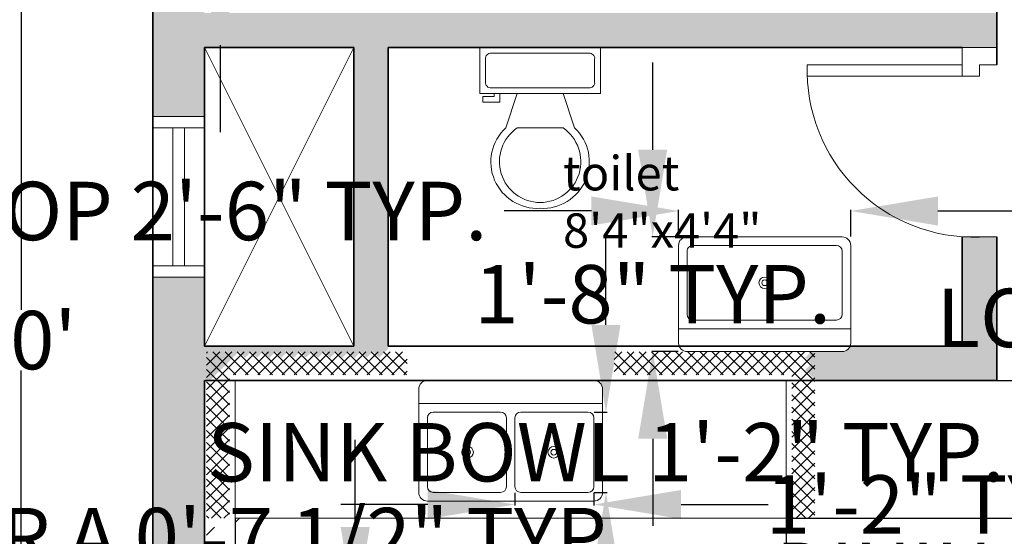
# Model space of a CAD drawing. Units: inches. Extents: x 19 to 15718, y 7 to 930.
# Tile 8 of 11: x 15243 to 15415, y 556 to 646. Entities that reach past the tile are written whole.
import ezdxf

# ---------------------------------------------------------------- set-up
doc = ezdxf.new("R2010")
doc.units = ezdxf.units.IN
doc.header["$MEASUREMENT"] = 0
for name, color, linetype, lineweight in [('A-ANNO-DIMS', 2, 'Continuous', 18), ('A-AREA-IDEN', 7, 'Continuous', 18), ('A-DOOR', 4, 'Continuous', 20), ('A-FLOR-CASE', 8, 'Continuous', 18), ('A-FLOR-CASE-PATT', 252, 'Continuous', 13), ('A-FLOR-FIXT', 9, 'Continuous', 18), ('A-FLOR-OPEN', 8, 'Continuous', 13), ('A-GLAZ', 4, 'Continuous', 18), ('A-WALL', 7, 'Continuous', 35)]:
    doc.layers.add(name, color=color, linetype=linetype, lineweight=lineweight)
doc.layers.add('A-WALL-PATT', color=18, linetype='Continuous', lineweight=13, true_color=0x000000)
doc.styles.add('Annotative', font='arial.ttf')
doc.styles.get("Standard").update_dxf_attribs({"font": 'arial.ttf'})
doc.dimstyles.get("Standard").update_dxf_attribs({"dimtxt": 10.18, "dimasz": 15.18, "dimexe": 0.18, "dimexo": 0.0625, "dimgap": 0.09, "dimtad": 0, "dimtih": 1, "dimtoh": 1, "dimdec": 0, "dimzin": 0, "dimdsep": 46, "dimlunit": 3, "dimtxsty": 'Standard', "dimcen": 0.09, "dimadec": 0, "dimazin": 0, "dimtfac": 1, "dimtdec": 0, "dimtofl": 0, "dimtmove": 0, "dimatfit": 3, "dimfxl": 1, "dimtolj": 1, "dimtzin": 0, "dimarcsym": 0})

# ---------------------------------------------------------------- blocks, each defined once
blk = doc.blocks.new('*U2')
for p, q in [((9.5, -6), (9.5, -2)), ((-10, -8.5), (-8, -8.5)), ((-10, -9.5), (-10, -8.5)), ((-8, -8.5), (-8, -8)), ((-7, -8), (-7, -9.5)), ((-4, -8), (-6, -14)), ((4, -8), (6, -14)), ((-7, -9.5), (-10, -9.5)), ((4, -14), (-4, -14))]:
    blk.add_line(p, q)
blk.add_lwpolyline([(10.5, -8), (10.5, 0), (-10.5, 0), (-10.5, -8)], close=True)
for points in [[(8.5, -1), (-8.5, -1)], [(-9.5, -2), (-9.5, -6)], [(-8.5, -7), (8.5, -7)]]:
    blk.add_lwpolyline(points)
for centre, radius, start, end in [((-8.625, -1.875), 0.8839, 81.8699, 188.1301), ((8.625, -1.875), 0.8839, 351.8699, 98.1301), ((-8.625, -6.125), 0.8839, 171.869898, 278.1301), ((8.625, -6.125), 0.8839, 261.8699, 8.1301), ((-0.4772, -19.9188), 8.0953, 133.01722, 273.38), ((0.0374, -19.8731), 7.127, 124.50543, 269.7), ((-0.0373, -19.8731), 7.127, 270.3, 55.4946), ((0.4773, -19.9188), 8.0953, 266.62, 46.9828)]:
    blk.add_arc(centre, radius, start, end)
blk = doc.blocks.new('*D17')
at = {"layer": 'A-ANNO-DIMS', "color": 0, "lineweight": -2, "transparency": 16777216}
for p, q in [((15266.62, 830.27), (15243.58, 830.27)), ((15243.76, 815.09), (15243.76, 595.52)), ((15243.76, 365.38), (15243.76, 584.95)), ((15266.62, 350.2), (15243.58, 350.2))]:
    blk.add_line(p, q, dxfattribs=at)
at = {"layer": 'A-ANNO-DIMS', "color": 0, "transparency": 16777216}
for points in [[(15241.23, 815.09), (15246.29, 815.09), (15243.76, 830.27)], [(15241.23, 365.38), (15246.29, 365.38), (15243.76, 350.2)]]:
    blk.add_solid(points, dxfattribs=at)
at = {"layer": 'Defpoints', "color": 0, "transparency": 16777216}
for p in [(15266.68, 830.27), (15243.76, 350.2), (15266.68, 350.2)]:
    blk.add_point(p, dxfattribs=at)
at = {"layer": 'A-ANNO-DIMS', "color": 0, "transparency": 16777216, "insert": (15243.76, 590.24), "char_height": 10.18, "attachment_point": 5}
blk.add_mtext("\\A1;40'", dxfattribs=at)
blk = doc.blocks.new('Sink-single - 30 in top')
blk.add_line((-15, -3.999996), (15, -3.999996))
for points in [[(-13.5, 0), (13.5, 0)], [(-15, -18.499996), (-15, -1.5)], [(15, -1.5), (15, -18.499996)], [(-13.5, -17.499996), (-13.5, -6.499996)], [(-12.5, -5.499996), (12.5, -5.499996)], [(13.5, -6.499996), (13.5, -17.499996)], [(12.5, -18.499996), (-12.5, -18.499996)], [(13.5, -19.999996), (-13.5, -19.999996)]]:
    blk.add_lwpolyline(points)
for radius in [1, 0.5]:
    blk.add_circle((0, -11.999996), radius)
for centre, radius, start, end in [((-13.5, -1.5), 1.5, 90, 180), ((13.5, -1.5), 1.5, 0, 90), ((-12.5, -6.499996), 1, 90, 180), ((12.5, -6.499996), 1, 0, 90), ((-13.5, -18.499996), 1.5, 180, 270), ((-12.5, -17.499996), 1, 180, 270), ((12.5, -17.499996), 1, 270, 0), ((13.5, -18.499996), 1.5, 270, 0)]:
    blk.add_arc(centre, radius, start, end)
blk = doc.blocks.new('DOOR-SWING-30IN')
for p, q in [((3, 6), (3, 33)), ((5, 3), (5, 33)), ((0, 6), (0, 0)), ((0, 6), (5, 6)), ((33, 6), (33, 0)), ((3, 3), (3, 0)), ((5, 3), (3, 3))]:
    blk.add_line(p, q)
blk.add_arc((4, 4), 29.02, 358.0251, 91.9749)
blk = doc.blocks.new('SINK-BOWL-14IN')
blk.add_line((0, 13), (0, 1))
for points in [[(1, 14), (12.75, 14)], [(13.75, 13), (13.75, 1)], [(12.75, 0), (1, 0)]]:
    blk.add_lwpolyline(points)
for radius in [1, 0.5]:
    blk.add_circle((6.75, 7), radius)
for centre, start, end in [((1, 13), 90, 180), ((12.75, 13), 0, 90), ((1, 1), 180, 270), ((12.75, 1), 270, 0)]:
    blk.add_arc(centre, 1, start, end)
blk = doc.blocks.new('*D40')
at = {"layer": 'A-ANNO-DIMS', "color": 0, "lineweight": -2, "transparency": 16777216}
for p, q in [((15117.25, 555.92), (15102.07, 555.92)), ((15132.43, 556.96), (15132.43, 555.74)), ((15139.78, 556.96), (15139.78, 555.74)), ((15154.96, 555.92), (15170.14, 555.92))]:
    blk.add_line(p, q, dxfattribs=at)
at = {"layer": 'A-ANNO-DIMS', "color": 0, "transparency": 16777216}
for points in [[(15117.25, 558.45), (15117.25, 553.39), (15132.43, 555.92)], [(15154.96, 558.45), (15154.96, 553.39), (15139.78, 555.92)]]:
    blk.add_solid(points, dxfattribs=at)
at = {"layer": 'Defpoints', "color": 0, "transparency": 16777216}
for p in [(15132.43, 557.02), (15139.78, 557.02), (15139.78, 555.92)]:
    blk.add_point(p, dxfattribs=at)
at = {"layer": 'A-ANNO-DIMS', "color": 0, "transparency": 16777216, "insert": (15262.49, 555.92), "char_height": 10.18, "attachment_point": 5}
blk.add_mtext('\\A1;SIDE CHAIR A 0\'-7 1/2" TYP.', dxfattribs=at)
blk = doc.blocks.new('*D42')
at = {"layer": 'A-ANNO-DIMS', "color": 0, "lineweight": -2, "transparency": 16777216}
for p, q in [((15133.17, 540.88), (15133.17, 542.1)), ((15140.52, 540.88), (15140.52, 542.1)), ((15117.99, 541.92), (15102.81, 541.92)), ((15155.7, 541.92), (15170.88, 541.92))]:
    blk.add_line(p, q, dxfattribs=at)
at = {"layer": 'A-ANNO-DIMS', "color": 0, "transparency": 16777216}
for points in [[(15117.99, 544.45), (15117.99, 539.39), (15133.17, 541.92)], [(15155.7, 544.45), (15155.7, 539.39), (15140.52, 541.92)]]:
    blk.add_solid(points, dxfattribs=at)
at = {"layer": 'Defpoints', "color": 0, "transparency": 16777216}
for p in [(15133.17, 540.82), (15140.52, 541.92), (15140.52, 540.82)]:
    blk.add_point(p, dxfattribs=at)
at = {"layer": 'A-ANNO-DIMS', "color": 0, "transparency": 16777216, "insert": (15263.22, 541.92), "char_height": 10.18, "attachment_point": 5}
blk.add_mtext('\\A1;SIDE CHAIR B 0\'-7 1/2" TYP.', dxfattribs=at)
blk = doc.blocks.new('*D46')
at = {"layer": 'A-ANNO-DIMS', "color": 0, "lineweight": -2, "transparency": 16777216}
for p, q in [((15343.07, 612.73), (15327.89, 612.73)), ((15358.25, 608.29), (15358.25, 612.91)), ((15388.25, 608.29), (15388.25, 612.91)), ((15403.43, 612.73), (15418.61, 612.73))]:
    blk.add_line(p, q, dxfattribs=at)
at = {"layer": 'A-ANNO-DIMS', "color": 0, "transparency": 16777216}
for points in [[(15343.07, 615.26), (15343.07, 610.2), (15358.25, 612.73)], [(15403.43, 615.26), (15403.43, 610.2), (15388.25, 612.73)]]:
    blk.add_solid(points, dxfattribs=at)
at = {"layer": 'Defpoints', "color": 0, "transparency": 16777216}
for p in [(15358.25, 612.73), (15358.25, 608.23), (15388.25, 608.23)]:
    blk.add_point(p, dxfattribs=at)
at = {"layer": 'A-ANNO-DIMS', "color": 0, "transparency": 16777216, "insert": (15257.09, 612.73), "char_height": 10.18, "attachment_point": 5}
blk.add_mtext('\\A1;BASIN TOP 2\'-6" TYP.', dxfattribs=at)
blk = doc.blocks.new('*D47')
at = {"layer": 'A-ANNO-DIMS', "color": 0, "lineweight": -2, "transparency": 16777216}
for p, q in [((15353.75, 623.41), (15353.75, 638.59)), ((15358.19, 608.23), (15353.57, 608.23)), ((15358.19, 588.23), (15353.57, 588.23)), ((15353.75, 573.05), (15353.75, 557.87))]:
    blk.add_line(p, q, dxfattribs=at)
at = {"layer": 'A-ANNO-DIMS', "color": 0, "transparency": 16777216}
for points in [[(15351.22, 623.41), (15356.28, 623.41), (15353.75, 608.23)], [(15351.22, 573.05), (15356.28, 573.05), (15353.75, 588.23)]]:
    blk.add_solid(points, dxfattribs=at)
at = {"layer": 'Defpoints', "color": 0, "transparency": 16777216}
for p in [(15358.25, 608.23), (15353.75, 588.23), (15358.25, 588.23)]:
    blk.add_point(p, dxfattribs=at)
at = {"layer": 'A-ANNO-DIMS', "color": 0, "transparency": 16777216, "insert": (15353.75, 598.23), "char_height": 10.18, "attachment_point": 5}
blk.add_mtext('\\A1;1\'-8" TYP.', dxfattribs=at)
blk = doc.blocks.new('*D57')
at = {"layer": 'A-ANNO-DIMS', "color": 0, "lineweight": -2, "transparency": 16777216}
for p, q in [((15165.53, 693.18), (15165.53, 708.36)), ((15165.53, 708.36), (15180.71, 708.36)), ((15166.82, 678), (15165.35, 678)), ((15166.82, 669.42), (15165.35, 669.42)), ((15165.53, 654.24), (15165.53, 639.06))]:
    blk.add_line(p, q, dxfattribs=at)
at = {"layer": 'A-ANNO-DIMS', "color": 0, "transparency": 16777216}
for points in [[(15163, 693.18), (15168.06, 693.18), (15165.53, 678)], [(15163, 654.24), (15168.06, 654.24), (15165.53, 669.42)]]:
    blk.add_solid(points, dxfattribs=at)
at = {"layer": 'Defpoints', "color": 0, "transparency": 16777216}
for p in [(15165.53, 678), (15166.88, 678), (15166.88, 669.42)]:
    blk.add_point(p, dxfattribs=at)
at = {"layer": 'A-ANNO-DIMS', "color": 0, "transparency": 16777216, "insert": (15223.69, 708.36), "char_height": 10.18, "attachment_point": 5}
blk.add_mtext('\\A1;0\'-8 1/2" TYP.', dxfattribs=at)
blk = doc.blocks.new('*D58')
at = {"layer": 'A-ANNO-DIMS', "color": 0, "lineweight": -2, "transparency": 16777216}
for p, q in [((15278.41, 688.79), (15278.41, 703.97)), ((15280.87, 673.61), (15278.23, 673.61)), ((15280.87, 656.82), (15278.23, 656.82)), ((15278.41, 641.64), (15278.41, 626.46))]:
    blk.add_line(p, q, dxfattribs=at)
at = {"layer": 'A-ANNO-DIMS', "color": 0, "transparency": 16777216}
for points in [[(15275.88, 688.79), (15280.94, 688.79), (15278.41, 673.61)], [(15275.88, 641.64), (15280.94, 641.64), (15278.41, 656.82)]]:
    blk.add_solid(points, dxfattribs=at)
at = {"layer": 'Defpoints', "color": 0, "transparency": 16777216}
for p in [(15278.41, 673.61), (15280.93, 673.61), (15280.93, 656.82)]:
    blk.add_point(p, dxfattribs=at)
at = {"layer": 'A-ANNO-DIMS', "color": 0, "transparency": 16777216, "insert": (15278.41, 665.21), "char_height": 10.18, "attachment_point": 5}
blk.add_mtext('\\A1;NIGHTSTAND 1\'-5" TYP.', dxfattribs=at)
blk = doc.blocks.new('*D66')
at = {"layer": 'A-ANNO-DIMS', "color": 0, "lineweight": -2, "transparency": 16777216}
for p, q in [((15345.61, 592.88), (15345.61, 608.06)), ((15343.57, 577.7), (15345.79, 577.7)), ((15343.57, 563.7), (15345.79, 563.7)), ((15345.61, 548.52), (15345.61, 533.34))]:
    blk.add_line(p, q, dxfattribs=at)
at = {"layer": 'A-ANNO-DIMS', "color": 0, "transparency": 16777216}
for points in [[(15343.08, 592.88), (15348.14, 592.88), (15345.61, 577.7)], [(15343.08, 548.52), (15348.14, 548.52), (15345.61, 563.7)]]:
    blk.add_solid(points, dxfattribs=at)
at = {"layer": 'Defpoints', "color": 0, "transparency": 16777216}
for p in [(15343.51, 577.7), (15345.61, 577.7), (15343.51, 563.7)]:
    blk.add_point(p, dxfattribs=at)
at = {"layer": 'A-ANNO-DIMS', "color": 0, "transparency": 16777216, "insert": (15345.61, 570.7), "char_height": 10.18, "attachment_point": 5}
blk.add_mtext('\\A1;SINK BOWL 1\'-2" TYP.', dxfattribs=at)
blk = doc.blocks.new('*D67')
at = {"layer": 'A-ANNO-DIMS', "color": 0, "lineweight": -2, "transparency": 16777216}
for p, q in [((15329.76, 563.64), (15329.76, 561.42)), ((15343.51, 563.64), (15343.51, 561.42)), ((15314.58, 561.6), (15299.4, 561.6)), ((15358.69, 561.6), (15373.87, 561.6))]:
    blk.add_line(p, q, dxfattribs=at)
at = {"layer": 'A-ANNO-DIMS', "color": 0, "transparency": 16777216}
for points in [[(15314.58, 564.13), (15314.58, 559.07), (15329.76, 561.6)], [(15358.69, 564.13), (15358.69, 559.07), (15343.51, 561.6)]]:
    blk.add_solid(points, dxfattribs=at)
at = {"layer": 'Defpoints', "color": 0, "transparency": 16777216}
for p in [(15329.76, 563.7), (15343.51, 563.7), (15343.51, 561.6)]:
    blk.add_point(p, dxfattribs=at)
at = {"layer": 'A-ANNO-DIMS', "color": 0, "transparency": 16777216, "insert": (15404.51, 561.6), "char_height": 10.18, "attachment_point": 5}
blk.add_mtext('\\A1;1\'-2" TYP.', dxfattribs=at)
blk = doc.blocks.new('*D68')
at = {"layer": 'A-ANNO-DIMS', "color": 0, "lineweight": -2, "transparency": 16777216}
for p, q in [((15309.3, 542.58), (15309.3, 550.07)), ((15324.48, 549.89), (15343.27, 549.89)), ((15358.45, 542.58), (15358.45, 550.07)), ((15358.45, 549.89), (15373.63, 549.89))]:
    blk.add_line(p, q, dxfattribs=at)
at = {"layer": 'A-ANNO-DIMS', "color": 0, "transparency": 16777216}
for points in [[(15324.48, 552.42), (15324.48, 547.36), (15309.3, 549.89)], [(15343.27, 552.42), (15343.27, 547.36), (15358.45, 549.89)]]:
    blk.add_solid(points, dxfattribs=at)
at = {"layer": 'Defpoints', "color": 0, "transparency": 16777216}
for p in [(15358.45, 549.89), (15309.3, 542.52), (15358.45, 542.52)]:
    blk.add_point(p, dxfattribs=at)
at = {"layer": 'A-ANNO-DIMS', "color": 0, "transparency": 16777216, "insert": (15429.66, 549.89), "char_height": 10.18, "attachment_point": 5}
blk.add_mtext('\\A1;DINING SET 4\'-1"', dxfattribs=at)
blk = doc.blocks.new('*D69')
at = {"layer": 'A-ANNO-DIMS', "color": 0, "lineweight": -2, "transparency": 16777216}
for p, q in [((15301.93, 557.7), (15301.93, 572.88)), ((15309.24, 542.52), (15301.75, 542.52)), ((15309.24, 512.82), (15301.75, 512.82)), ((15301.93, 497.64), (15301.93, 482.46))]:
    blk.add_line(p, q, dxfattribs=at)
at = {"layer": 'A-ANNO-DIMS', "color": 0, "transparency": 16777216}
for points in [[(15299.4, 557.7), (15304.46, 557.7), (15301.93, 542.52)], [(15299.4, 497.64), (15304.46, 497.64), (15301.93, 512.82)]]:
    blk.add_solid(points, dxfattribs=at)
at = {"layer": 'Defpoints', "color": 0, "transparency": 16777216}
for p in [(15301.93, 542.52), (15309.3, 542.52), (15309.3, 512.82)]:
    blk.add_point(p, dxfattribs=at)
at = {"layer": 'A-ANNO-DIMS', "color": 0, "transparency": 16777216, "insert": (15301.93, 527.67), "char_height": 10.18, "attachment_point": 5}
blk.add_mtext('\\A1;2\'-5 1/2"', dxfattribs=at)
blk = doc.blocks.new('*D72')
at = {"layer": 'A-ANNO-DIMS', "color": 0, "lineweight": -2, "transparency": 16777216}
for p, q in [((15548.36, 643.79), (15553.66, 643.79)), ((15553.48, 628.61), (15553.48, 624.46)), ((15548.36, 609.28), (15553.66, 609.28)), ((15553.48, 609.28), (15553.48, 594.1)), ((15553.48, 594.1), (15538.3, 594.1))]:
    blk.add_line(p, q, dxfattribs=at)
at = {"layer": 'A-ANNO-DIMS', "color": 0, "transparency": 16777216}
for points in [[(15550.95, 628.61), (15556.01, 628.61), (15553.48, 643.79)], [(15550.95, 624.46), (15556.01, 624.46), (15553.48, 609.28)]]:
    blk.add_solid(points, dxfattribs=at)
at = {"layer": 'Defpoints', "color": 0, "transparency": 16777216}
for p in [(15548.3, 643.79), (15548.3, 609.28), (15553.48, 609.28)]:
    blk.add_point(p, dxfattribs=at)
at = {"layer": 'A-ANNO-DIMS', "color": 0, "transparency": 16777216, "insert": (15469.57, 594.1), "char_height": 10.18, "attachment_point": 5}
blk.add_mtext('\\A1;LOVESEAT 2\'-10 1/2"', dxfattribs=at)
blk = doc.blocks.new('*D81')
at = {"layer": 'A-ANNO-DIMS', "color": 0, "lineweight": -2, "transparency": 16777216}
for p, q in [((15281.01, 559.14), (15281.01, 314.67)), ((15377.01, 559.14), (15377.01, 314.67)), ((15296.19, 314.85), (15315.38, 314.85)), ((15361.83, 314.85), (15342.64, 314.85))]:
    blk.add_line(p, q, dxfattribs=at)
at = {"layer": 'A-ANNO-DIMS', "color": 0, "transparency": 16777216}
for points in [[(15296.19, 317.38), (15296.19, 312.32), (15281.01, 314.85)], [(15361.83, 317.38), (15361.83, 312.32), (15377.01, 314.85)]]:
    blk.add_solid(points, dxfattribs=at)
at = {"layer": 'Defpoints', "color": 0, "transparency": 16777216}
for p in [(15281.01, 559.2), (15377.01, 559.2), (15377.01, 314.85)]:
    blk.add_point(p, dxfattribs=at)
at = {"layer": 'A-ANNO-DIMS', "color": 0, "transparency": 16777216, "insert": (15329.01, 314.85), "char_height": 10.18, "attachment_point": 5}
blk.add_mtext('\\A1;8\'-0"', dxfattribs=at)
blk = doc.blocks.new('*D82')
at = {"layer": 'A-ANNO-DIMS', "color": 0, "lineweight": -2, "transparency": 16777216}
for p, q in [((15602.030581, 598.383955), (15602.030581, 613.563955)), ((15377.073779, 583.203955), (15602.210581, 583.203955)), ((15377.073779, 559.203955), (15602.210581, 559.203955)), ((15602.030581, 544.023955), (15602.030581, 528.843955))]:
    blk.add_line(p, q, dxfattribs=at)
at = {"layer": 'A-ANNO-DIMS', "color": 0, "transparency": 16777216}
for points in [[(15599.500581, 598.383955), (15604.560581, 598.383955), (15602.030581, 583.203955)], [(15599.500581, 544.023955), (15604.560581, 544.023955), (15602.030581, 559.203955)]]:
    blk.add_solid(points, dxfattribs=at)
at = {"layer": 'Defpoints', "color": 0, "transparency": 16777216}
for p in [(15377.011279, 583.203955), (15602.030581, 583.203955), (15377.011279, 559.203955)]:
    blk.add_point(p, dxfattribs=at)
at = {"layer": 'A-ANNO-DIMS', "color": 0, "transparency": 16777216, "insert": (15602.030581, 571.203955), "char_height": 10.18, "attachment_point": 5}
blk.add_mtext('\\A1;2\'-0"', dxfattribs=at)

msp = doc.modelspace()

# ---------------------------------------------------------------- hatches: boundary and pattern name
at = {"layer": 'A-FLOR-CASE-PATT'}
h = msp.add_hatch(dxfattribs=at)
h.set_pattern_fill('ANSI37', color=256, scale=12, style=0)
h.paths.add_polyline_path([(15276.01, 559.2), (15280.01, 559.2), (15280.01, 584.2), (15311.01, 584.2), (15311.01, 588.2), (15276.01, 588.2)])
h = msp.add_hatch(dxfattribs=at)
h.set_pattern_fill('ANSI37', color=256, scale=12, style=0)
h.paths.add_polyline_path([(15347.01, 588.2), (15347.01, 584.2), (15378.01, 584.2), (15378.01, 559.2), (15382.01, 559.2), (15382.01, 588.2)])
at = {"layer": 'A-WALL-PATT'}
h = msp.add_hatch(color=256, dxfattribs=at)
h.dxf.hatch_style = 1
h.paths.add_polyline_path([(15190.84, 837), (14890.84, 837), (14890.84, 357), (14899.84, 357), (14899.84, 366), (14899.84, 528), (14904.84, 528), (14904.84, 534), (14899.84, 534), (14899.84, 698), (15004.84, 698), (15004.84, 701, -0.014283), (15004.84, 703), (15004.84, 704), (14899.84, 704), (14899.84, 828), (14987.26, 828), (15043.84, 828), (15049.84, 828), (15075.84, 828), (15081.84, 828), (15181.84, 828), (15181.84, 780), (15114.84, 780), (15114.84, 779, -0.017236), (15114.84, 777), (15114.84, 774), (15181.84, 774), (15181.84, 654), (15181.84, 648), (15181.84, 596), (15190.84, 596)])
h.paths.add_polyline_path([(15190.84, 590), (15181.84, 590), (15181.84, 470), (15181.84, 464), (15181.84, 361.43), (14991.9, 361.43), (14991.5, 357), (15190.84, 357)], flags=0)
h.paths.add_polyline_path([(15152.29, 608), (15146.29, 608), (15146.29, 596), (15049.84, 596), (15049.84, 590), (15152.29, 590)], flags=17)
h.paths.add_polyline_path([(15049.84, 615), (15048.84, 615, -0.017236), (15046.84, 615), (15043.84, 615), (15043.84, 596), (15049.84, 596)], flags=17)
edge = h.paths.add_edge_path(flags=17)
edge.add_line((15152.29, 654), (15049.84, 654))
edge.add_line((15049.84, 654), (15043.84, 654))
edge.add_line((15043.84, 654), (15043.84, 648))
edge.add_line((15043.84, 648), (15049.84, 648))
edge.add_line((15049.84, 648), (15075.84, 648))
edge.add_line((15075.84, 648), (15081.84, 648))
edge.add_line((15081.84, 648), (15117.26, 648))
edge.add_spline(control_points=[(15117.26, 648), (15117.59, 648.02), (15117.94, 648.03), (15118.71, 648.04), (15119.15, 648.02), (15119.59, 648)], knot_values=[1.499122, 1.499122, 1.499122, 1.499122, 1.618335, 1.618335, 1.770388, 1.770388, 1.770388, 1.770388], degree=3, periodic=0)
edge.add_spline(control_points=[(15127.99, 642.93), (15128, 643.28), (15127.95, 643.62), (15127.73, 644.26), (15127.57, 644.57), (15127.16, 645.13), (15126.92, 645.39), (15126.04, 646.16), (15125.28, 646.6), (15123.53, 647.31), (15122.55, 647.59), (15120.88, 647.88), (15120.24, 647.95), (15119.59, 648)], knot_values=[0, 0, 0, 0, 0.172075, 0.172075, 0.344149, 0.344149, 0.516224, 0.516224, 0.894541, 0.894541, 1.272858, 1.272858, 1.499122, 1.499122, 1.499122, 1.499122], degree=3, periodic=0)
edge.add_line((15119.59, 648), (15146.29, 648))
edge.add_line((15146.29, 648), (15146.29, 636))
edge.add_line((15146.29, 636), (15152.29, 636))
edge.add_line((15152.29, 636), (15152.29, 654))
h.paths.add_polyline_path([(15132.35, 430.4), (15123.35, 430.4), (15123.35, 396.8), (15027.77, 396.8), (15027.77, 387.8), (15132.35, 387.8)], flags=17)
h.paths.add_polyline_path([(15132.35, 464), (15123.35, 464), (15123.35, 430.4), (15132.35, 430.4)], flags=17)
h.paths.add_polyline_path([(15275.68, 583.59), (15276.07, 583.2), (15276.65, 583.2), (15280.6, 587.16), (15278.55, 589.2), (15275.68, 589.2), (15275.68, 601.2), (15266.68, 601.2), (15266.68, 350.2), (15275.68, 350.2), (15275.68, 359.2), (15275.68, 457.2), (15413.68, 457.2), (15413.68, 471.04), (15407.68, 471.04), (15407.68, 463.2), (15275.68, 463.2)])
h = msp.add_hatch(color=256, dxfattribs=at)
h.dxf.hatch_style = 1
h.paths.add_polyline_path([(15566.68, 830.2), (15266.68, 830.2), (15266.68, 629.2), (15275.68, 629.2), (15275.68, 641.2), (15301.68, 641.2), (15301.68, 589.2), (15275.68, 589.2), (15275.68, 601.2), (15266.68, 601.2), (15266.68, 350.2), (15275.68, 350.2), (15275.68, 359.2), (15275.68, 457.2), (15413.68, 457.2), (15413.68, 471.04), (15407.68, 471.04), (15407.68, 463.2), (15275.68, 463.2), (15275.68, 583.59), (15276.07, 583.2), (15276.65, 583.2), (15277.42, 583.97), (15276.36, 585.03), (15279.54, 588.22), (15280.6, 587.16), (15281.66, 588.22), (15282.72, 587.16), (15283.78, 588.22), (15284.85, 587.16), (15285.91, 588.22), (15286.97, 587.16), (15288.03, 588.22), (15289.09, 587.16), (15290.15, 588.22), (15291.21, 587.16), (15292.27, 588.22), (15293.33, 587.16), (15294.39, 588.22), (15295.45, 587.16), (15296.51, 588.22), (15297.57, 587.16), (15298.63, 588.22), (15299.69, 587.16), (15300.76, 588.22), (15301.82, 587.16), (15302.88, 588.22), (15303.94, 587.16), (15305, 588.22), (15306.06, 587.16), (15307.68, 588.78), (15307.68, 641.2), (15407.68, 641.2), (15413.68, 641.2), (15413.68, 647.2), (15407.68, 647.2), (15275.68, 647.2), (15275.68, 767.2), (15336.68, 767.2), (15336.68, 773.2), (15275.68, 773.2), (15275.68, 821.2), (15375.68, 821.2), (15381.68, 821.2), (15407.68, 821.2), (15413.68, 821.2), (15557.68, 821.2), (15557.68, 697.2), (15452.68, 697.2), (15452.68, 696.2, -0.014283), (15452.68, 694.2), (15452.68, 691.2), (15557.68, 691.2), (15557.68, 527.2), (15557.68, 521.2), (15557.68, 359.2), (15557.68, 350.2), (15566.68, 350.2)])
h.paths.add_polyline_path([(15416.63, 527.2), (15413.68, 527.2), (15407.68, 527.2), (15407.68, 521.04), (15413.68, 521.04), (15413.68, 521.2), (15416.63, 521.2)], flags=17)
h.paths.add_polyline_path([(15432.13, 393.97), (15308.13, 393.97), (15308.13, 425.59), (15299.13, 425.59), (15299.13, 384.97), (15432.13, 384.97)], flags=17)
h.paths.add_polyline_path([(15308.13, 457.2), (15299.13, 457.2), (15299.13, 425.59), (15308.13, 425.59)], flags=17)
h.paths.add_polyline_path([(15425.57, 359.2), (15275.68, 359.2), (15275.68, 350.2), (15425.57, 350.2)], flags=17)
h.paths.add_polyline_path([(15413.68, 797.2), (15407.68, 797.2), (15407.68, 773.2), (15381.68, 773.2), (15381.68, 797.2), (15375.68, 797.2), (15375.68, 773.2), (15375.68, 767.2), (15407.68, 767.2), (15407.68, 686.2), (15408.68, 686.2, -0.014283), (15410.68, 686.2), (15413.68, 686.2), (15413.68, 691.2), (15413.68, 697.2)], flags=17)
h.paths.add_polyline_path([(15413.68, 608.2), (15410.68, 608.2, -0.017236), (15408.68, 608.2), (15407.68, 608.2), (15407.68, 589.2), (15388.16, 589.2, -0.313626), (15386.75, 588.23), (15381.37, 588.23), (15380.3, 587.16), (15381.37, 586.1), (15380.3, 585.03), (15382.14, 583.2), (15407.68, 583.2), (15413.68, 583.2)], flags=17)

# ---------------------------------------------------------------- linework, layer by layer
at = {"layer": 'A-FLOR-CASE'}
for p, q in [((15281.01, 583.2), (15377.01, 583.2)), ((15281.01, 559.2), (15281.01, 583.2)), ((15377.01, 583.2), (15377.01, 559.2)), ((15377.01, 559.2), (15281.01, 559.2))]:
    msp.add_line(p, q, dxfattribs=at)
at = {"layer": 'A-FLOR-CASE-PATT'}
for p, q in [((15281.76, 559.2), (15281.01, 558.45)), ((15277.41, 557.66), (15276.01, 556.26))]:
    msp.add_line(p, q, dxfattribs=at)
at = {"layer": 'A-FLOR-FIXT'}
msp.add_line((15313.01, 579.2), (15345.01, 579.2), dxfattribs=at)
for points in [[(15314.51, 583.2), (15343.51, 583.2)], [(15313.01, 563.7), (15313.01, 581.7)], [(15345.01, 581.7), (15345.01, 563.7)], [(15343.51, 562.2), (15314.51, 562.2)]]:
    msp.add_lwpolyline(points, dxfattribs=at)
for centre, start, end in [((15314.51, 581.7), 90, 180), ((15343.51, 581.7), 0, 90), ((15314.51, 563.7), 180, 270), ((15343.51, 563.7), 270, 0)]:
    msp.add_arc(centre, 1.5, start, end, dxfattribs=at)
at = {"layer": 'A-FLOR-OPEN'}
for p, q in [((15275.68, 641.2), (15301.68, 589.2)), ((15301.68, 641.2), (15275.68, 589.2))]:
    msp.add_line(p, q, dxfattribs=at)
at = {"layer": 'A-GLAZ'}
for p, q in [((15275.68, 629.2), (15266.68, 629.2)), ((15275.68, 627.2), (15266.68, 627.2)), ((15270.18, 627.2), (15270.18, 603.2)), ((15272.18, 627.2), (15272.18, 603.2)), ((15275.68, 603.2), (15266.68, 603.2)), ((15275.68, 601.2), (15266.68, 601.2))]:
    msp.add_line(p, q, dxfattribs=at)
at = {"layer": 'A-WALL'}
for p, q in [((15266.68, 350.2), (15266.68, 830.2)), ((15413.68, 650.2), (15413.68, 638.2)), ((15275.68, 641.2), (15301.68, 641.2)), ((15275.68, 589.2), (15275.68, 641.2)), ((15301.68, 641.2), (15301.68, 589.2)), ((15307.68, 641.2), (15307.68, 589.2)), ((15307.68, 641.2), (15407.68, 641.2)), ((15407.68, 608.26), (15407.68, 589.2)), ((15413.68, 608.2), (15413.68, 583.2)), ((15275.68, 589.2), (15301.68, 589.2)), ((15307.68, 589.2), (15407.68, 589.2)), ((15275.68, 583.2), (15407.68, 583.2)), ((15275.68, 463.2), (15275.68, 583.2)), ((15407.68, 583.2), (15413.68, 583.2))]:
    msp.add_line(p, q, dxfattribs=at)

# ---------------------------------------------------------------- block references
at = {"layer": 'A-DOOR', "extrusion": (0, 0, -1), "zscale": -1, "rotation": 269.9999999999902}
msp.add_blockref('DOOR-SWING-30IN', (-15413.68, 641.2), dxfattribs=at)
at = {"layer": 'A-FLOR-FIXT'}
for name, p in [('*U2', (15334.14, 641.2)), ('SINK-BOWL-14IN', (15329.76, 563.7))]:
    msp.add_blockref(name, p, dxfattribs=at)
at = {"layer": 'A-FLOR-FIXT', "rotation": 180}
msp.add_blockref('Sink-single - 30 in top', (15373.25, 588.23), dxfattribs=at)
at = {"layer": 'A-FLOR-FIXT', "extrusion": (0, 0, -1), "zscale": -1}
msp.add_blockref('SINK-BOWL-14IN', (-15328.26, 563.7), dxfattribs=at)

# ---------------------------------------------------------------- texts
at = {"layer": 'A-AREA-IDEN', "insert": (15338.14, 622.32), "char_height": 6, "width": 68.1983, "attachment_point": 1, "style": 'Annotative'}
msp.add_mtext('toilet\\P8\'4"x4\'4"', dxfattribs=at)

# ---------------------------------------------------------------- dimensions: what is measured, and where the dimension line sits
at = {"layer": 'A-ANNO-DIMS'}
for base, p1, p2, override, picture, middle in [((15243.76, 350.2), (15266.68, 830.27), (15266.68, 350.2), {"dimclrd": 0, "dimclre": 0, "dimclrt": 0}, '*D17', (15243.76, 590.24)), ((15602.03, 583.2), (15377.01, 559.2), (15377.01, 583.2), {"dimdec": 1, "dimlfac": 1, "dimrnd": 0, "dimzin": 1, "dimdsep": 46, "dimlunit": 4, "dimfrac": 2}, '*D82', (15602.03, 571.2)), ((15301.93, 542.52), (15309.3, 512.82), (15309.3, 542.52), {"dimdec": 1, "dimlfac": 1, "dimrnd": 0, "dimzin": 1, "dimdsep": 46, "dimlunit": 4, "dimfrac": 2}, '*D69', (15301.93, 527.67))]:
    dim = msp.add_linear_dim(base=base, p1=p1, p2=p2, angle=90, dimstyle='Standard', override=override, dxfattribs=at)
    dim.commit()
    dim.dimension.update_dxf_attribs({"geometry": picture, "text_midpoint": middle})
for base, p1, p2, angle, text, picture, middle in [((15165.53, 678), (15166.88, 669.42), (15166.88, 678), 90, '<> TYP.', '*D57', (15223.69, 708.36)), ((15278.41, 673.61), (15280.93, 656.82), (15280.93, 673.61), 90, 'NIGHTSTAND <> TYP.', '*D58', (15278.41, 665.21)), ((15358.25, 612.73), (15388.25, 608.23), (15358.25, 608.23), 180, 'BASIN TOP <> TYP.', '*D46', (15257.09, 612.73)), ((15553.48, 609.28), (15548.3, 643.79), (15548.3, 609.28), 270, 'LOVESEAT <>', '*D72', (15469.57, 594.1)), ((15353.75, 588.23), (15358.25, 608.23), (15358.25, 588.23), 270, '<> TYP.', '*D47', (15353.75, 598.23)), ((15345.61, 577.7), (15343.51, 563.7), (15343.51, 577.7), 90, 'SINK BOWL <> TYP.', '*D66', (15345.61, 570.7))]:
    dim = msp.add_linear_dim(base=base, p1=p1, p2=p2, angle=angle, text=text, dimstyle='Standard', override={"dimdec": 1, "dimlfac": 1, "dimrnd": 0, "dimzin": 1, "dimdsep": 46, "dimlunit": 4, "dimfrac": 2}, dxfattribs=at)
    dim.commit()
    dim.dimension.update_dxf_attribs({"geometry": picture, "text_midpoint": middle})
for base, p1, p2, text, picture, middle in [((15139.7848, 555.9195), (15132.4322, 557.0224), (15139.7848, 557.0224), 'SIDE CHAIR A <> TYP.', '*D40', (15262.4867, 555.9195)), ((15140.519, 541.924), (15133.1663, 540.8211), (15140.519, 540.8211), 'SIDE CHAIR B <> TYP.', '*D42', (15263.2209, 541.924)), ((15343.51127927, 561.60395495), (15329.76127927, 563.70395495), (15343.51127927, 563.70395495), '<> TYP.', '*D67', (15404.50822333, 561.60395495)), ((15358.4492, 549.8921), (15309.3028, 542.5201), (15358.4492, 542.5201), 'DINING SET <>', '*D68', (15429.664, 549.8921))]:
    dim = msp.add_linear_dim(base=base, p1=p1, p2=p2, text=text, dimstyle='Standard', override={"dimdec": 1, "dimlfac": 1, "dimrnd": 0, "dimzin": 1, "dimdsep": 46, "dimlunit": 4, "dimfrac": 2}, dxfattribs=at)
    dim.commit()
    dim.dimension.update_dxf_attribs({"geometry": picture, "text_midpoint": middle})
dim = msp.add_linear_dim(base=(15377.01, 314.85), p1=(15281.01, 559.2), p2=(15377.01, 559.2), dimstyle='Standard', override={"dimdec": 1, "dimlfac": 1, "dimrnd": 0, "dimzin": 1, "dimdsep": 46, "dimlunit": 4, "dimfrac": 2}, dxfattribs=at)
dim.commit()
dim.dimension.update_dxf_attribs({"geometry": '*D81', "text_midpoint": (15329.01, 314.85)})

doc.saveas('drawing.dxf')
